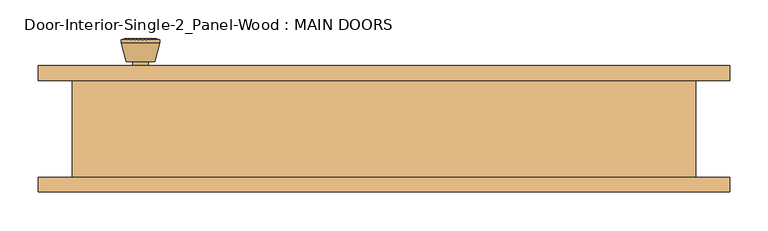
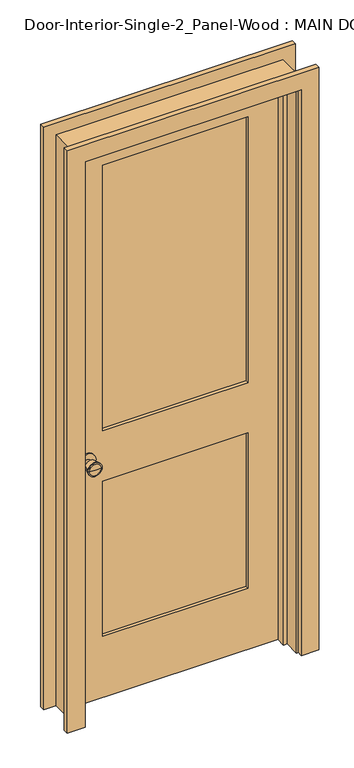
"""IFC4 building model written with IfcOpenShell, lengths in millimetres: door geometry, Door-Interior-Single-2_Panel-Wood : MAIN DOORS."""

from ifc_helpers import new_model, si_unit, point, frame, frame_2d, origin, place, context, project, spatial, polyline, circle_curve, trimmed, segment, composite_curve, outline, extrude, faceted_brep, source, transform, mapped, element, save
from ifc_brep_helpers import plane_surface, cylinder_surface, revolved_surface, advanced_brep


def door_interior_single_2_panel_wood_main_doors_a5f98f63(model_context):
    return source(origin(), model_context, "Body", "SolidModel", [
        advanced_brep(
        [(-317.5, 19.4, 914.4), (-307.5, 19.4, 914.4), (-327.5, 19.4, 914.4), (-297.0241324, -29.6, 914.4), (-317.5, -29.6, 914.4), (-337.9758676, -29.6, 914.4), (-292.5, -27.7721319, 914.4), (-342.5, -27.7721319, 914.4), (-292.5, -24.3084537, 914.4), (-342.5, -24.3084537, 914.4), (-298.863764, 0.4, 914.4), (-336.136236, 0.4, 914.4), (-307.5, 0.4, 914.4), (-327.5, 0.4, 914.4)],
        [
            (0, 1),
            (1, 2, circle_curve(frame((-317.5, 19.4, 914.4), z_axis=(0.0, 1.0, 0.0), x_axis=(-1.0, 0.0, 0.0)), 10.0)),
            (2, 0),
            (2, 1, circle_curve(frame((-317.5, 19.4, 914.4), z_axis=(0.0, 1.0, 0.0), x_axis=(-1.0, 0.0, 0.0)), 10.0)),
            (3, 4),
            (4, 5),
            (5, 3, circle_curve(frame((-317.5, -29.6, 914.4), z_axis=(0.0, -1.0, 0.0), x_axis=(-1.0, 0.0, 0.0)), 20.4758676)),
            (3, 5, circle_curve(frame((-317.5, -29.6, 914.4), z_axis=(0.0, -1.0, 0.0), x_axis=(-1.0, 0.0, 0.0)), 20.4758676)),
            (6, 3),
            (5, 7),
            (7, 6, circle_curve(frame((-317.5, -27.7721319, 914.4), z_axis=(0.0, -1.0, 0.0), x_axis=(-1.0, 0.0, 0.0)), 25.0)),
            (6, 7, circle_curve(frame((-317.5, -27.7721319, 914.4), z_axis=(0.0, -1.0, 0.0), x_axis=(-1.0, 0.0, 0.0)), 25.0)),
            (8, 6),
            (7, 9),
            (9, 8, circle_curve(frame((-317.5, -24.3084537, 914.4), z_axis=(0.0, -1.0, 0.0), x_axis=(-1.0, 0.0, 0.0)), 25.0)),
            (8, 9, circle_curve(frame((-317.5, -24.3084537, 914.4), z_axis=(0.0, -1.0, 0.0), x_axis=(-1.0, 0.0, 0.0)), 25.0)),
            (10, 8),
            (9, 11),
            (11, 10, circle_curve(frame((-317.5, 0.4, 914.4), z_axis=(0.0, -1.0, 0.0), x_axis=(-1.0, 0.0, 0.0)), 18.636236)),
            (10, 11, circle_curve(frame((-317.5, 0.4, 914.4), z_axis=(0.0, -1.0, 0.0), x_axis=(-1.0, 0.0, 0.0)), 18.636236)),
            (12, 10),
            (11, 13),
            (13, 12, circle_curve(frame((-317.5, 0.4, 914.4), z_axis=(0.0, -1.0, 0.0), x_axis=(-1.0, 0.0, 0.0)), 10.0)),
            (12, 13, circle_curve(frame((-317.5, 0.4, 914.4), z_axis=(0.0, -1.0, 0.0), x_axis=(-1.0, 0.0, 0.0)), 10.0)),
            (1, 12),
            (13, 2),
        ],
        [
            plane_surface(frame((-317.5, 19.4, 914.4), z_axis=(0.0, 1.0, 0.0), x_axis=(-1.0, 0.0, 0.0))),
            plane_surface(frame((-317.5, -29.6, 914.4), z_axis=(0.0, -1.0, 0.0), x_axis=(-1.0, 0.0, 0.0))),
            revolved_surface(polyline([(-337.9758676, -29.6, 914.4), (-342.5, -27.7721319, 914.4)]), (-317.5, 19.4, 914.4), (0.0, 1.0, 0.0)),
            cylinder_surface(frame((-317.5, 19.4, 914.4), z_axis=(0.0, 1.0, 0.0), x_axis=(-1.0, 0.0, 0.0)), 25.0),
            revolved_surface(polyline([(-342.5, -24.3084537, 914.4), (-336.136236, 0.4, 914.4)]), (-317.5, 19.4, 914.4), (0.0, 1.0, 0.0)),
            plane_surface(frame((-317.5, 0.4, 914.4), z_axis=(0.0, 1.0, 0.0), x_axis=(-1.0, 0.0, 0.0))),
            cylinder_surface(frame((-317.5, 19.4, 914.4), z_axis=(0.0, 1.0, 0.0), x_axis=(-1.0, 0.0, 0.0)), 10.0),
        ],
        [
            (0, [[1, 2, 3]]),
            (0, [[-3, 4, -1]]),
            (1, [[5, 6, 7]]),
            (1, [[-6, -5, 8]]),
            (2, [[9, -7, 10, 11]]),
            (2, [[-10, -8, -9, 12]]),
            (3, [[13, -11, 14, 15]]),
            (3, [[-14, -12, -13, 16]]),
            (4, [[17, -15, 18, 19]]),
            (4, [[-18, -16, -17, 20]]),
            (5, [[21, -19, 22, 23]]),
            (5, [[-22, -20, -21, 24]]),
            (6, [[25, -23, 26, -2]]),
            (6, [[-26, -24, -25, -4]]),
        ],
    ),
        extrude(outline(composite_curve([segment(trimmed(circle_curve(frame_2d((914.4, -317.5)), 30.0), [point((914.4, -347.5))], [point((914.4, -287.5))], False, "CARTESIAN"), True, "CONTINUOUS"), segment(trimmed(circle_curve(frame_2d((914.4, -317.5)), 30.0), [point((914.4, -287.5))], [point((914.4, -347.5))], False, "CARTESIAN"), True, "CONTINUOUS")], self_intersect=False)), frame((0.0, 19.4, 0.0), z_axis=(0.0, 1.0, 0.0), x_axis=(0.0, 0.0, 1.0)), (0.0, 0.0, 1.0), 6.0),
        advanced_brep(
        [(-317.5, 66.325, 914.4), (-327.5, 66.325, 914.4), (-307.5, 66.325, 914.4), (-297.0241324, 115.325, 914.4), (-337.9758676, 115.325, 914.4), (-317.5, 115.325, 914.4), (-292.5, 113.4971319, 914.4), (-342.5, 113.4971319, 914.4), (-292.5, 110.0334537, 914.4), (-342.5, 110.0334537, 914.4), (-298.863764, 85.325, 914.4), (-336.136236, 85.325, 914.4), (-307.5, 85.325, 914.4), (-327.5, 85.325, 914.4)],
        [
            (0, 1),
            (1, 2, circle_curve(frame((-317.5, 66.325, 914.4), z_axis=(0.0, -1.0, 0.0), x_axis=(-1.0, 0.0, 0.0)), 10.0)),
            (2, 0),
            (2, 1, circle_curve(frame((-317.5, 66.325, 914.4), z_axis=(0.0, -1.0, 0.0), x_axis=(-1.0, 0.0, 0.0)), 10.0)),
            (3, 4, circle_curve(frame((-317.5, 115.325, 914.4), z_axis=(0.0, 1.0, 0.0), x_axis=(-1.0, 0.0, 0.0)), 20.4758676)),
            (4, 5),
            (5, 3),
            (4, 3, circle_curve(frame((-317.5, 115.325, 914.4), z_axis=(0.0, 1.0, 0.0), x_axis=(-1.0, 0.0, 0.0)), 20.4758676)),
            (6, 7, circle_curve(frame((-317.5, 113.4971319, 914.4), z_axis=(0.0, 1.0, 0.0), x_axis=(-1.0, 0.0, 0.0)), 25.0)),
            (7, 4),
            (3, 6),
            (7, 6, circle_curve(frame((-317.5, 113.4971319, 914.4), z_axis=(0.0, 1.0, 0.0), x_axis=(-1.0, 0.0, 0.0)), 25.0)),
            (8, 9, circle_curve(frame((-317.5, 110.0334537, 914.4), z_axis=(0.0, 1.0, 0.0), x_axis=(-1.0, 0.0, 0.0)), 25.0)),
            (9, 7),
            (6, 8),
            (9, 8, circle_curve(frame((-317.5, 110.0334537, 914.4), z_axis=(0.0, 1.0, 0.0), x_axis=(-1.0, 0.0, 0.0)), 25.0)),
            (10, 11, circle_curve(frame((-317.5, 85.325, 914.4), z_axis=(0.0, 1.0, 0.0), x_axis=(-1.0, 0.0, 0.0)), 18.636236)),
            (11, 9),
            (8, 10),
            (11, 10, circle_curve(frame((-317.5, 85.325, 914.4), z_axis=(0.0, 1.0, 0.0), x_axis=(-1.0, 0.0, 0.0)), 18.636236)),
            (12, 13, circle_curve(frame((-317.5, 85.325, 914.4), z_axis=(0.0, 1.0, 0.0), x_axis=(-1.0, 0.0, 0.0)), 10.0)),
            (13, 11),
            (10, 12),
            (13, 12, circle_curve(frame((-317.5, 85.325, 914.4), z_axis=(0.0, 1.0, 0.0), x_axis=(-1.0, 0.0, 0.0)), 10.0)),
            (1, 13),
            (12, 2),
        ],
        [
            plane_surface(frame((-317.5, 66.325, 914.4), z_axis=(0.0, -1.0, 0.0), x_axis=(-1.0, 0.0, 0.0))),
            plane_surface(frame((-317.5, 115.325, 914.4), z_axis=(0.0, 1.0, 0.0), x_axis=(-1.0, 0.0, 0.0))),
            revolved_surface(polyline([(-337.9758676, 115.325, 914.4), (-342.5, 113.4971319, 914.4)]), (-317.5, 66.325, 914.4), (0.0, -1.0, 0.0)),
            cylinder_surface(frame((-317.5, 66.325, 914.4), z_axis=(0.0, -1.0, 0.0), x_axis=(-1.0, 0.0, 0.0)), 25.0),
            revolved_surface(polyline([(-342.5, 110.0334537, 914.4), (-336.136236, 85.325, 914.4)]), (-317.5, 66.325, 914.4), (0.0, -1.0, 0.0)),
            plane_surface(frame((-317.5, 85.325, 914.4), z_axis=(0.0, -1.0, 0.0), x_axis=(-1.0, 0.0, 0.0))),
            cylinder_surface(frame((-317.5, 66.325, 914.4), z_axis=(0.0, -1.0, 0.0), x_axis=(-1.0, 0.0, 0.0)), 10.0),
        ],
        [
            (0, [[1, 2, 3]]),
            (0, [[-3, 4, -1]]),
            (1, [[5, 6, 7]]),
            (1, [[8, -7, -6]]),
            (2, [[9, 10, -5, 11]]),
            (2, [[12, -11, -8, -10]]),
            (3, [[13, 14, -9, 15]]),
            (3, [[16, -15, -12, -14]]),
            (4, [[17, 18, -13, 19]]),
            (4, [[20, -19, -16, -18]]),
            (5, [[21, 22, -17, 23]]),
            (5, [[24, -23, -20, -22]]),
            (6, [[-2, 25, -21, 26]]),
            (6, [[-4, -26, -24, -25]]),
        ],
    ),
        extrude(outline(composite_curve([segment(trimmed(circle_curve(frame_2d((914.4, -317.5)), 30.0), [point((914.4, -347.5))], [point((914.4, -287.5))], False, "CARTESIAN"), True, "CONTINUOUS"), segment(trimmed(circle_curve(frame_2d((914.4, -317.5)), 30.0), [point((914.4, -287.5))], [point((914.4, -347.5))], False, "CARTESIAN"), True, "CONTINUOUS")], self_intersect=False)), frame((0.0, 60.325, 0.0), z_axis=(0.0, 1.0, 0.0), x_axis=(0.0, 0.0, 1.0)), (0.0, 0.0, 1.0), 6.0),
        faceted_brep([(406.4, 60.325, 0.0), (406.4, -66.675, 0.0), (381.0, -66.675, 0.0), (381.0, -9.525, 0.0), (368.3, -9.525, 0.0), (368.3, 25.4, 0.0), (381.0, 25.4, 0.0), (381.0, 60.325, 0.0), (406.4, 60.325, 2159.0), (406.4, -66.675, 2159.0), (-406.4, -66.675, 2159.0), (-406.4, -66.675, 0.0), (-381.0, -66.675, 0.0), (-381.0, -66.675, 2133.6), (381.0, -66.675, 2133.6), (381.0, -9.525, 2133.6), (-381.0, -9.525, 2133.6), (-381.0, -9.525, 0.0), (-368.3, -9.525, 0.0), (-368.3, -9.525, 2120.9), (368.3, -9.525, 2120.9), (368.3, 25.4, 2120.9), (-368.3, 25.4, 2120.9), (-368.3, 25.4, 0.0), (-381.0, 25.4, 0.0), (-381.0, 25.4, 2133.6), (381.0, 25.4, 2133.6), (381.0, 60.325, 2133.6), (-381.0, 60.325, 2133.6), (-381.0, 60.325, 0.0), (-406.4, 60.325, 0.0), (-406.4, 60.325, 2159.0)], [[[0, 1, 2, 3, 4, 5, 6, 7]], [[1, 0, 8, 9]], [[2, 1, 9, 10, 11, 12, 13, 14]], [[3, 2, 14, 15]], [[4, 3, 15, 16, 17, 18, 19, 20]], [[5, 4, 20, 21]], [[6, 5, 21, 22, 23, 24, 25, 26]], [[7, 6, 26, 27]], [[0, 7, 27, 28, 29, 30, 31, 8]], [[9, 8, 31, 10]], [[15, 14, 13, 16]], [[21, 20, 19, 22]], [[27, 26, 25, 28]], [[30, 29, 24, 23, 18, 17, 12, 11]], [[10, 31, 30, 11]], [[16, 13, 12, 17]], [[22, 19, 18, 23]], [[28, 25, 24, 29]]]),
        extrude(outline(polyline([(2133.6, -381.0), (0.0, -381.0), (0.0, 381.0), (2133.6, 381.0), (2133.6, -381.0)]), holes=[polyline([(2014.5375, -260.35), (2014.5375, 260.35), (1009.65, 260.35), (1009.65, -260.35), (2014.5375, -260.35)]), polyline([(819.15, -260.35), (819.15, 260.35), (231.775, 260.35), (231.775, -260.35), (819.15, -260.35)])]), frame((0.0, 25.4, 0.0), z_axis=(0.0, 1.0, 0.0), x_axis=(0.0, 0.0, 1.0)), (0.0, 0.0, 1.0), 34.925),
        extrude(outline(polyline([(260.35, 37.0416667), (-260.35, 37.0416667), (-260.35, 48.6833333), (260.35, 48.6833333), (260.35, 37.0416667)])), frame((0.0, 0.0, 1009.65), z_axis=(0.0, 0.0, 1.0), x_axis=(1.0, 0.0, 0.0)), (0.0, 0.0, 1.0), 1004.8875),
        extrude(outline(polyline([(260.35, 37.0416667), (-260.35, 37.0416667), (-260.35, 48.6833333), (260.35, 48.6833333), (260.35, 37.0416667)])), frame((0.0, 0.0, 231.775), z_axis=(0.0, 0.0, 1.0), x_axis=(1.0, 0.0, 0.0)), (0.0, 0.0, 1.0), 587.375),
        extrude(outline(polyline([(0.0, 387.35), (0.0, 450.85), (2203.45, 450.85), (2203.45, -450.85), (0.0, -450.85), (0.0, -387.35), (2139.95, -387.35), (2139.95, 387.35), (0.0, 387.35)])), frame((0.0, 60.325, 0.0), z_axis=(0.0, 1.0, 0.0), x_axis=(0.0, 0.0, 1.0)), (0.0, 0.0, 1.0), 19.05),
        extrude(outline(polyline([(0.0, 387.35), (0.0, 450.85), (2203.45, 450.85), (2203.45, -450.85), (0.0, -450.85), (0.0, -387.35), (2139.95, -387.35), (2139.95, 387.35), (0.0, 387.35)])), frame((0.0, -85.725, 0.0), z_axis=(0.0, 1.0, 0.0), x_axis=(0.0, 0.0, 1.0)), (0.0, 0.0, 1.0), 19.05),
    ])


if __name__ == "__main__":
    model = new_model("IFC4")
    model_context = context("Model", 3, world=origin())
    ifc_project = project(units=[si_unit("LENGTHUNIT", "METRE", prefix="MILLI")], contexts=[model_context])
    site = spatial("IfcSite", under=ifc_project)
    building = spatial("IfcBuilding", under=site)
    placement = place(None, origin())
    door_interior_single_2_panel_wood_main_doors_shape = door_interior_single_2_panel_wood_main_doors_a5f98f63(model_context)
    element("IfcDoor", 1, ObjectType="Door-Interior-Single-2_Panel-Wood : MAIN DOORS", at=placement, inside=building, context=model_context, shape_type="MappedRepresentation", body=[
        mapped(door_interior_single_2_panel_wood_main_doors_shape, transform((0.0, 0.0, 0.0), x_axis=(1.0, 0.0, 0.0), y_axis=(0.0, 1.0, 0.0), z_axis=(0.0, 0.0, 1.0))),
    ])
    save(model, "model.ifc")

# Revit data of these elements
# Type "Door-Interior-Single-2_Panel-Wood : MAIN DOORS"
#   Type Mark = "10"
#   Assembly Code = "C1020300"
#   Analytic Construction = "Wooden"
#   Top Rail = 0' - 4 11/16"
#   Thickness = 0' - 1 3/8"
#   Thermal Resistance (R) = 2.5876 (h·ft²·°F)/BTU
#   Swing Angle [instance default] = 90.00°
#   Stiles = 0' - 4 3/4"
#   Rough Width = 2' - 8"
#   Rough Height = 7' - 1"
#   Lock Rail = 0' - 7 1/2"
#   Height = 7' - 0"
#   Width = 2' - 6"
#   Heat Transfer Coefficient (U) = 0.3865 BTU/(h·ft²·°F)
#   Bottom Rail = 0' - 9 1/8"
#   Trim Material = Cherry
#   Panel Material = Cherry
#   Frame Material = Cherry
#   Door Handle Material = Aluminum
#   Visual Light Transmittance = 0
#   Solar Heat Gain Coefficient = 0
#   Wall Closure = (empty or 0)
#   Function = (empty or 0)
# Element 1 (IfcDoor, "Door-Interior-Single-2_Panel-Wood : MAIN DOORS")
#   Materials on its faces: "Cherry", "Aluminum"
# Materials
#   "Cherry": class "Wood", colour RGB 226 177 128, transparency 0, Description = "Prunus Serotina", Cost = 0
#   "Aluminum": class "Metal", colour RGB 247 247 247, transparency 0, Description = "Aluminum 6061", Cost = 0
